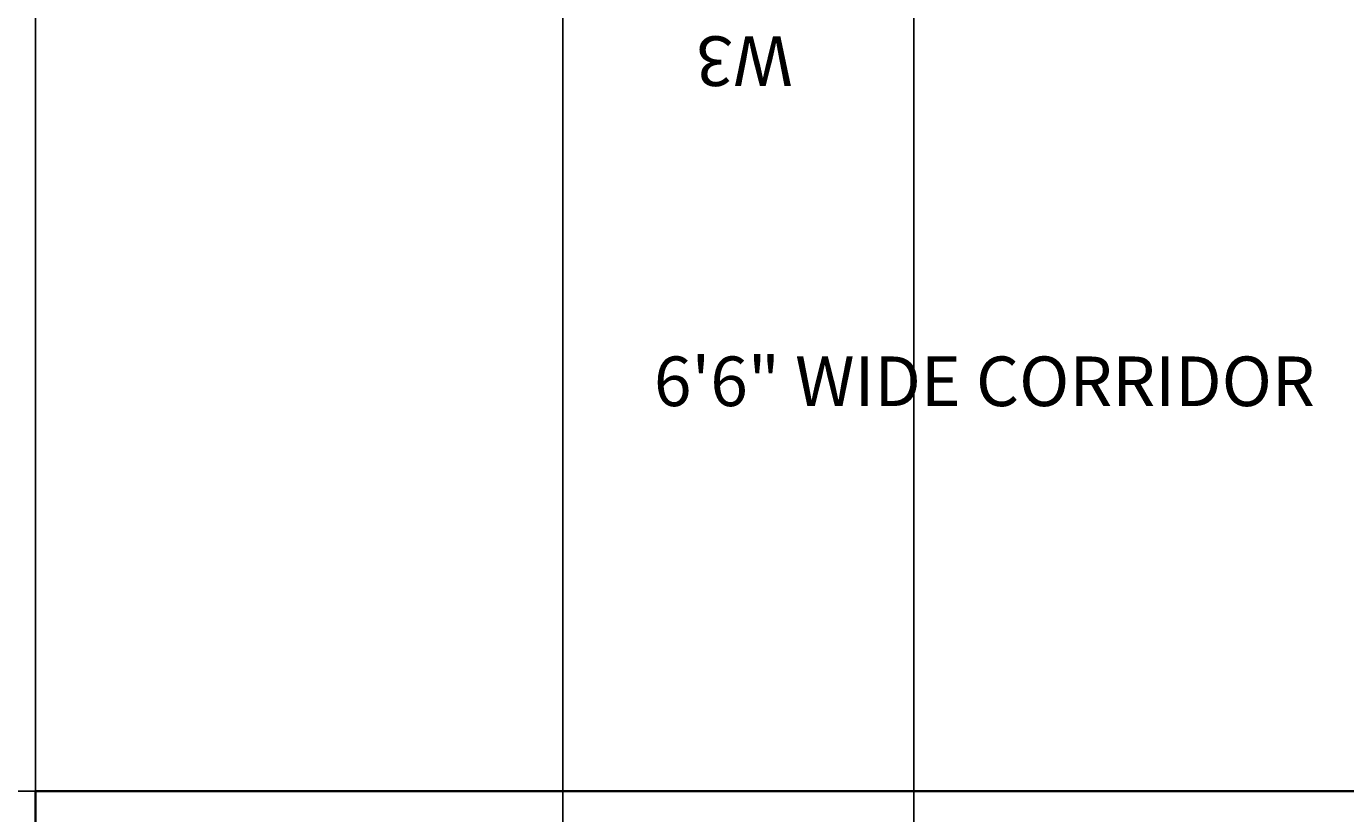
# Model space of a CAD drawing. Units: inches. Extents: x -86 to 2463, y -1058 to 68.
# Tile 4 of 17: x 15 to 148, y -383 to -304. Entities that reach past the tile are written whole.
import ezdxf

# ---------------------------------------------------------------- set-up
doc = ezdxf.new("R2010")
doc.units = ezdxf.units.IN
doc.header["$MEASUREMENT"] = 0
for name, color, linetype, lineweight in [('A-ANNO-DIMS', 2, 'Continuous', 18), ('A-ANNO-TEXT', 7, 'Continuous', 18), ('A-AREA-IDEN', 7, 'Continuous', 18), ('A-WALL', 7, 'Continuous', 35)]:
    doc.layers.add(name, color=color, linetype=linetype, lineweight=lineweight)
doc.styles.get("Standard").update_dxf_attribs({"font": 'arial.ttf'})
doc.dimstyles.get("Standard").update_dxf_attribs({"dimtxt": 0.18, "dimasz": 0.18, "dimexe": 0.18, "dimexo": 0.0625, "dimgap": 0.09, "dimtad": 0, "dimtih": 1, "dimtoh": 1, "dimdec": 4, "dimzin": 0, "dimdsep": 46, "dimtxsty": 'Standard', "dimcen": 0.09, "dimadec": 0, "dimazin": 0, "dimtfac": 1, "dimtdec": 4, "dimtofl": 0, "dimtmove": 0, "dimatfit": 3, "dimfxl": 1, "dimtolj": 1, "dimtzin": 0, "dimarcsym": 0})

# ---------------------------------------------------------------- blocks, each defined once
blk = doc.blocks.new('*D33')
at = {"layer": 'A-ANNO-DIMS', "color": 0, "lineweight": -2, "transparency": 16777216}
for p, q in [((15.7, -381.1), (-86.02, -381.1)), ((-85.84, -381.28), (-85.84, -504.09)), ((-85.84, -627.25), (-85.84, -504.45)), ((15.7, -627.43), (-86.02, -627.43))]:
    blk.add_line(p, q, dxfattribs=at)
at = {"layer": 'A-ANNO-DIMS', "color": 0, "transparency": 16777216}
for points in [[(-85.87, -381.28), (-85.81, -381.28), (-85.84, -381.1)], [(-85.87, -627.25), (-85.81, -627.25), (-85.84, -627.43)]]:
    blk.add_solid(points, dxfattribs=at)
at = {"layer": 'Defpoints', "color": 0, "transparency": 16777216}
for p in [(-85.84, -381.1), (15.76, -381.1), (15.76, -627.43)]:
    blk.add_point(p, dxfattribs=at)
at = {"layer": 'A-ANNO-DIMS', "color": 0, "transparency": 16777216, "insert": (-85.84, -504.27), "char_height": 0.18, "attachment_point": 5}
blk.add_mtext('\\A1;246.33', dxfattribs=at)
blk = doc.blocks.new('*D41')
at = {"layer": 'A-ANNO-DIMS', "color": 0, "lineweight": -2, "transparency": 16777216}
for p, q in [((15.76, -303.17), (15.76, -740.38)), ((68.89, -303.17), (68.89, -740.38)), ((15.94, -740.2), (41.93, -740.2)), ((68.71, -740.2), (42.72, -740.2))]:
    blk.add_line(p, q, dxfattribs=at)
at = {"layer": 'A-ANNO-DIMS', "color": 0, "transparency": 16777216}
for points in [[(15.94, -740.17), (15.94, -740.23), (15.76, -740.2)], [(68.71, -740.17), (68.71, -740.23), (68.89, -740.2)]]:
    blk.add_solid(points, dxfattribs=at)
at = {"layer": 'Defpoints', "color": 0, "transparency": 16777216}
for p in [(15.76, -303.1), (68.89, -303.1), (68.89, -740.2)]:
    blk.add_point(p, dxfattribs=at)
at = {"layer": 'A-ANNO-DIMS', "color": 0, "transparency": 16777216, "insert": (42.33, -740.2), "char_height": 0.18, "attachment_point": 5}
blk.add_mtext('\\A1;53.13', dxfattribs=at)
blk = doc.blocks.new('*D42')
at = {"layer": 'A-ANNO-DIMS', "color": 0, "lineweight": -2, "transparency": 16777216}
for p, q in [((68.89, -303.17), (68.89, -740.38)), ((104.26, -303.17), (104.26, -740.38)), ((69.07, -740.2), (86.18, -740.2)), ((104.08, -740.2), (86.97, -740.2))]:
    blk.add_line(p, q, dxfattribs=at)
at = {"layer": 'A-ANNO-DIMS', "color": 0, "transparency": 16777216}
for points in [[(69.07, -740.17), (69.07, -740.23), (68.89, -740.2)], [(104.08, -740.17), (104.08, -740.23), (104.26, -740.2)]]:
    blk.add_solid(points, dxfattribs=at)
at = {"layer": 'Defpoints', "color": 0, "transparency": 16777216}
for p in [(68.89, -303.1), (104.26, -303.1), (104.26, -740.2)]:
    blk.add_point(p, dxfattribs=at)
at = {"layer": 'A-ANNO-DIMS', "color": 0, "transparency": 16777216, "insert": (86.58, -740.2), "char_height": 0.18, "attachment_point": 5}
blk.add_mtext('\\A1;35.37', dxfattribs=at)

msp = doc.modelspace()

# ---------------------------------------------------------------- linework, layer by layer
at = {"layer": 'A-WALL'}
for p, q in [((377.846, -381.104), (15.761, -381.104)), ((15.761, -381.104), (15.761, -627.432))]:
    msp.add_line(p, q, dxfattribs=at)

# ---------------------------------------------------------------- texts
at = {"layer": 'A-ANNO-TEXT', "insert": (92.062, -310.027), "char_height": 5, "attachment_point": 1, "rotation": 180}
msp.add_mtext_dynamic_manual_height_columns('W3', width=36.57058, gutter_width=25, heights=[0], dxfattribs=at)
at = {"layer": 'A-AREA-IDEN', "insert": (78.08, -337.287), "char_height": 5, "attachment_point": 1}
msp.add_mtext_dynamic_manual_height_columns('6\'6" WIDE CORRIDOR', width=176.45231, gutter_width=25, heights=[0], dxfattribs=at)

# ---------------------------------------------------------------- dimensions: what is measured, and where the dimension line sits
at = {"layer": 'A-ANNO-DIMS'}
for base, p1, p2, picture, middle in [((68.889, -740.204), (15.761, -303.104), (68.889, -303.104), '*D41', (42.325, -740.204)), ((104.261, -740.204), (68.889, -303.104), (104.261, -303.104), '*D42', (86.575, -740.204))]:
    dim = msp.add_linear_dim(base=base, p1=p1, p2=p2, dimstyle='Standard', override={"dimdec": 2, "dimlfac": 1, "dimrnd": 0, "dimzin": 0, "dimdsep": 46, "dimlunit": 2}, dxfattribs=at)
    dim.commit()
    dim.dimension.update_dxf_attribs({"geometry": picture, "text_midpoint": middle})
dim = msp.add_linear_dim(base=(-85.839, -381.104), p1=(15.761, -627.432), p2=(15.761, -381.104), angle=90, dimstyle='Standard', override={"dimdec": 2, "dimlfac": 1, "dimrnd": 0, "dimzin": 0, "dimdsep": 46, "dimlunit": 2}, dxfattribs=at)
dim.commit()
dim.dimension.update_dxf_attribs({"geometry": '*D33', "text_midpoint": (-85.839, -504.268)})

doc.saveas('drawing.dxf')
